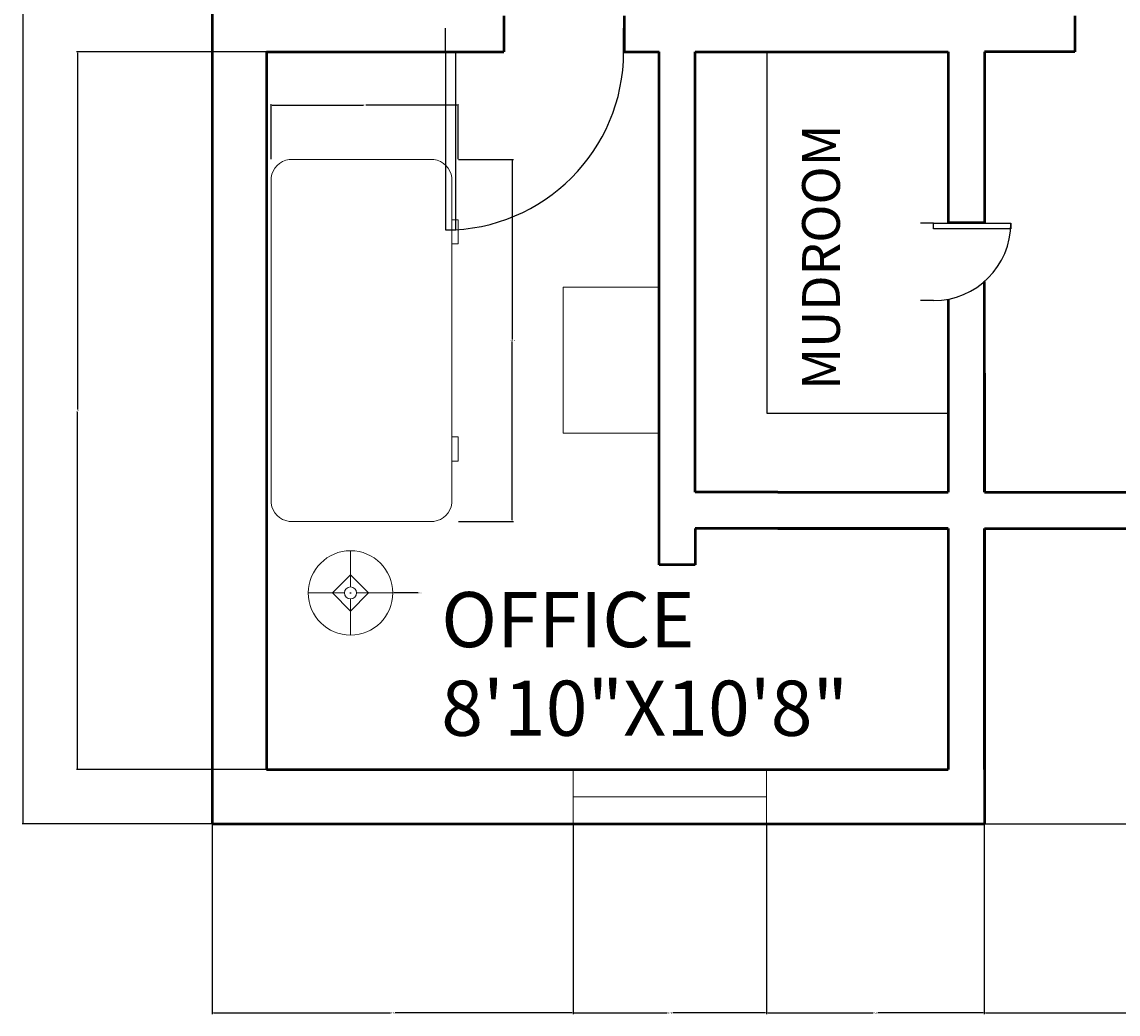
# Model space of a CAD drawing. Units: inches. Extents: x 2208 to 4689, y 1219 to 3512.
# Tile 1 of 5: x 2208 to 2389, y 1219 to 1383. Entities that reach past the tile are written whole.
import ezdxf

# ---------------------------------------------------------------- set-up
doc = ezdxf.new("R2010")
doc.units = ezdxf.units.IN
for name, color, linetype, lineweight in [('A-ANNO-DIMS', 2, 'Continuous', 18), ('A-AREA-IDEN', 7, 'Continuous', 18), ('A-DOOR', 3, 'Continuous', 25), ('A-FLOR-CASE', 9, 'Continuous', 25), ('A-FURN', 8, 'Continuous', 18), ('A-GLAZ', 4, 'Continuous', 18), ('A-WALL', 7, 'Continuous', 50)]:
    doc.layers.add(name, color=color, linetype=linetype, lineweight=lineweight)
doc.styles.get("Standard").update_dxf_attribs({"font": 'arial.ttf'})
doc.dimstyles.get("Standard").update_dxf_attribs({"dimtxt": 0.18, "dimasz": 0.18, "dimexe": 0.18, "dimexo": 0.0625, "dimgap": 0.09, "dimtad": 0, "dimtih": 1, "dimtoh": 1, "dimdec": 4, "dimzin": 0, "dimdsep": 46, "dimtxsty": 'Standard', "dimcen": 0.09, "dimadec": 0, "dimazin": 0, "dimtfac": 1, "dimtdec": 4, "dimtofl": 0, "dimtmove": 0, "dimatfit": 3, "dimfxl": 1, "dimtolj": 1, "dimtzin": 0, "dimarcsym": 0})

# ---------------------------------------------------------------- blocks, each defined once
blk = doc.blocks.new('*U15')
for p, q in [((0, 0), (0, -100)), ((600, 0), (600, -100))]:
    blk.add_line(p, q)
blk.add_lwpolyline([(0, 0), (0, 600), (43.75, 600), (43.75, 0)], close=True)
blk.add_arc((0, 0), 600, 0, 90)
blk = doc.blocks.new('Lamp - Table')
for p, q in [((0, 7), (0, 1)), ((0, 3), (-3, 0)), ((3, 0), (0, 3)), ((-1, 0), (-7, 0)), ((-3, 0), (0, -3)), ((0, -3), (3, 0)), ((1, 0), (7, 0)), ((0, -1), (0, -7))]:
    blk.add_line(p, q)
for radius in [7, 1]:
    blk.add_circle((0, 0), radius)
blk = doc.blocks.new('Desk - 30 x 60 in.')
for p, q in [((-26.999995, 0), (26.999995, 0)), ((-29.999995, -27), (-29.999995, -3)), ((29.999995, -3), (29.999995, -27)), ((26.999995, -30), (-26.999995, -30)), ((-20.000005, -30), (-20.000005, -31)), ((-16.000005, -31), (-16.000005, -30)), ((15.999995, -31), (15.999995, -30)), ((19.999995, -30), (19.999995, -31)), ((-20.000005, -31), (-16.000005, -31)), ((19.999995, -31), (15.999995, -31))]:
    blk.add_line(p, q)
for centre, start, end in [((-26.499995, -3.5), 98.1301, 171.8699), ((26.499995, -3.5), 8.130102, 81.8699), ((-26.499995, -26.5), 188.1301, 261.8699), ((26.499995, -26.5), 278.1301, 351.8699)]:
    blk.add_arc(centre, 3.535534, start, end)
blk = doc.blocks.new('*U4')
for p, q in [((0, 0), (0, 100)), ((750, 0), (750, 100))]:
    blk.add_line(p, q)
blk.add_lwpolyline([(0, 0), (0, -750), (43.75, -750), (43.75, 0)], close=True)
blk.add_arc((0, 0), 750, 270, 0)
blk = doc.blocks.new('*D26')
at = {"layer": 'A-ANNO-DIMS', "color": 0, "lineweight": -2, "transparency": 16777216}
for p, q in [((2279.91, 1360.51), (2289.03, 1360.51)), ((2288.85, 1360.33), (2288.85, 1330.69)), ((2288.85, 1300.69), (2288.85, 1330.32)), ((2279.91, 1300.51), (2289.03, 1300.51))]:
    blk.add_line(p, q, dxfattribs=at)
at = {"layer": 'A-ANNO-DIMS', "color": 0, "transparency": 16777216}
for points in [[(2288.82, 1360.33), (2288.88, 1360.33), (2288.85, 1360.51)], [(2288.82, 1300.69), (2288.88, 1300.69), (2288.85, 1300.51)]]:
    blk.add_solid(points, dxfattribs=at)
at = {"layer": 'Defpoints', "color": 0, "transparency": 16777216}
for p in [(2279.85, 1360.51), (2288.85, 1360.51), (2279.85, 1300.51)]:
    blk.add_point(p, dxfattribs=at)
at = {"layer": 'A-ANNO-DIMS', "color": 0, "transparency": 16777216, "insert": (2288.85, 1330.51), "char_height": 0.18, "attachment_point": 5}
blk.add_mtext('\\A1;DESK 60', dxfattribs=at)
blk = doc.blocks.new('*D27')
at = {"layer": 'A-ANNO-DIMS', "color": 0, "lineweight": -2, "transparency": 16777216}
for p, q in [((2248.85, 1360.57), (2248.85, 1369.69)), ((2249.03, 1369.51), (2264.15, 1369.51)), ((2279.67, 1369.51), (2264.55, 1369.51)), ((2279.85, 1360.57), (2279.85, 1369.69))]:
    blk.add_line(p, q, dxfattribs=at)
at = {"layer": 'A-ANNO-DIMS', "color": 0, "transparency": 16777216}
for points in [[(2249.03, 1369.54), (2249.03, 1369.48), (2248.85, 1369.51)], [(2279.67, 1369.54), (2279.67, 1369.48), (2279.85, 1369.51)]]:
    blk.add_solid(points, dxfattribs=at)
at = {"layer": 'Defpoints', "color": 0, "transparency": 16777216}
for p in [(2248.85, 1369.51), (2248.85, 1360.51), (2279.85, 1360.51)]:
    blk.add_point(p, dxfattribs=at)
at = {"layer": 'A-ANNO-DIMS', "color": 0, "transparency": 16777216, "insert": (2264.35, 1369.51), "char_height": 0.18, "attachment_point": 5}
blk.add_mtext('\\A1;31', dxfattribs=at)
blk = doc.blocks.new('*D35')
at = {"layer": 'A-ANNO-DIMS', "color": 0, "lineweight": -2, "transparency": 16777216}
for p, q in [((2239.04, 1850.36), (2207.57, 1850.36)), ((2207.75, 1850.18), (2207.75, 1550.54)), ((2207.75, 1250.54), (2207.75, 1550.17)), ((2239.04, 1250.36), (2207.57, 1250.36))]:
    blk.add_line(p, q, dxfattribs=at)
at = {"layer": 'A-ANNO-DIMS', "color": 0, "transparency": 16777216}
for points in [[(2207.72, 1850.18), (2207.78, 1850.18), (2207.75, 1850.36)], [(2207.72, 1250.54), (2207.78, 1250.54), (2207.75, 1250.36)]]:
    blk.add_solid(points, dxfattribs=at)
at = {"layer": 'Defpoints', "color": 0, "transparency": 16777216}
for p in [(2207.75, 1850.36), (2239.1, 1850.36), (2239.1, 1250.36)]:
    blk.add_point(p, dxfattribs=at)
at = {"layer": 'A-ANNO-DIMS', "color": 0, "transparency": 16777216, "insert": (2207.75, 1550.36), "char_height": 0.18, "attachment_point": 5}
blk.add_mtext('\\A1;600', dxfattribs=at)
blk = doc.blocks.new('*D40')
at = {"layer": 'A-ANNO-DIMS', "color": 0, "lineweight": -2, "transparency": 16777216}
for p, q in [((2248.04, 1378.36), (2216.57, 1378.36)), ((2216.75, 1378.18), (2216.75, 1319.04)), ((2216.75, 1259.54), (2216.75, 1318.67)), ((2248.04, 1259.36), (2216.57, 1259.36))]:
    blk.add_line(p, q, dxfattribs=at)
at = {"layer": 'A-ANNO-DIMS', "color": 0, "transparency": 16777216}
for points in [[(2216.72, 1378.18), (2216.78, 1378.18), (2216.75, 1378.36)], [(2216.72, 1259.54), (2216.78, 1259.54), (2216.75, 1259.36)]]:
    blk.add_solid(points, dxfattribs=at)
at = {"layer": 'Defpoints', "color": 0, "transparency": 16777216}
for p in [(2216.75, 1378.36), (2248.1, 1378.36), (2248.1, 1259.36)]:
    blk.add_point(p, dxfattribs=at)
at = {"layer": 'A-ANNO-DIMS', "color": 0, "transparency": 16777216, "insert": (2216.75, 1318.86), "char_height": 0.18, "attachment_point": 5}
blk.add_mtext('\\A1;119', dxfattribs=at)
blk = doc.blocks.new('*D47')
at = {"layer": 'A-ANNO-DIMS', "color": 0, "lineweight": -2, "transparency": 16777216}
for p, q in [((2239.1, 1250.29), (2239.1, 1218.83)), ((2298.94, 1250.29), (2298.94, 1218.83)), ((2239.28, 1219.01), (2268.63, 1219.01)), ((2298.76, 1219.01), (2269.41, 1219.01))]:
    blk.add_line(p, q, dxfattribs=at)
at = {"layer": 'A-ANNO-DIMS', "color": 0, "transparency": 16777216}
for points in [[(2239.28, 1219.04), (2239.28, 1218.98), (2239.1, 1219.01)], [(2298.76, 1219.04), (2298.76, 1218.98), (2298.94, 1219.01)]]:
    blk.add_solid(points, dxfattribs=at)
at = {"layer": 'Defpoints', "color": 0, "transparency": 16777216}
for p in [(2239.1, 1250.36), (2298.94, 1250.36), (2298.94, 1219.01)]:
    blk.add_point(p, dxfattribs=at)
at = {"layer": 'A-ANNO-DIMS', "color": 0, "transparency": 16777216, "insert": (2269.02, 1219.01), "char_height": 0.18, "attachment_point": 5}
blk.add_mtext('\\A1;59.84', dxfattribs=at)
blk = doc.blocks.new('*D48')
at = {"layer": 'A-ANNO-DIMS', "color": 0, "lineweight": -2, "transparency": 16777216}
for p, q in [((2298.94, 1250.29), (2298.94, 1218.83)), ((2331.01, 1250.29), (2331.01, 1218.83)), ((2299.12, 1219.01), (2314.51, 1219.01)), ((2330.83, 1219.01), (2315.44, 1219.01))]:
    blk.add_line(p, q, dxfattribs=at)
at = {"layer": 'A-ANNO-DIMS', "color": 0, "transparency": 16777216}
for points in [[(2299.12, 1219.04), (2299.12, 1218.98), (2298.94, 1219.01)], [(2330.83, 1219.04), (2330.83, 1218.98), (2331.01, 1219.01)]]:
    blk.add_solid(points, dxfattribs=at)
at = {"layer": 'Defpoints', "color": 0, "transparency": 16777216}
for p in [(2298.94, 1250.36), (2331.01, 1250.36), (2331.01, 1219.01)]:
    blk.add_point(p, dxfattribs=at)
at = {"layer": 'A-ANNO-DIMS', "color": 0, "transparency": 16777216, "insert": (2314.97, 1219.01), "char_height": 0.18, "attachment_point": 5}
blk.add_mtext('\\A1;32.064', dxfattribs=at)
blk = doc.blocks.new('*D49')
at = {"layer": 'A-ANNO-DIMS', "color": 0, "lineweight": -2, "transparency": 16777216}
for p, q in [((2331.01, 1250.29), (2331.01, 1218.83)), ((2367.11, 1250.29), (2367.11, 1218.83)), ((2331.19, 1219.01), (2348.68, 1219.01)), ((2366.93, 1219.01), (2349.44, 1219.01))]:
    blk.add_line(p, q, dxfattribs=at)
at = {"layer": 'A-ANNO-DIMS', "color": 0, "transparency": 16777216}
for points in [[(2331.19, 1219.04), (2331.19, 1218.98), (2331.01, 1219.01)], [(2366.93, 1219.04), (2366.93, 1218.98), (2367.11, 1219.01)]]:
    blk.add_solid(points, dxfattribs=at)
at = {"layer": 'Defpoints', "color": 0, "transparency": 16777216}
for p in [(2331.01, 1250.36), (2367.11, 1250.36), (2367.11, 1219.01)]:
    blk.add_point(p, dxfattribs=at)
at = {"layer": 'A-ANNO-DIMS', "color": 0, "transparency": 16777216, "insert": (2349.06, 1219.01), "char_height": 0.18, "attachment_point": 5}
blk.add_mtext('\\A1;36.11', dxfattribs=at)
blk = doc.blocks.new('*D50')
at = {"layer": 'A-ANNO-DIMS', "color": 0, "lineweight": -2, "transparency": 16777216}
for p, q in [((2367.11, 1299.29), (2367.11, 1218.83)), ((2427.95, 1299.29), (2427.95, 1218.83)), ((2367.29, 1219.01), (2397.14, 1219.01)), ((2427.77, 1219.01), (2397.93, 1219.01))]:
    blk.add_line(p, q, dxfattribs=at)
at = {"layer": 'A-ANNO-DIMS', "color": 0, "transparency": 16777216}
for points in [[(2367.29, 1219.04), (2367.29, 1218.98), (2367.11, 1219.01)], [(2427.77, 1219.04), (2427.77, 1218.98), (2427.95, 1219.01)]]:
    blk.add_solid(points, dxfattribs=at)
at = {"layer": 'Defpoints', "color": 0, "transparency": 16777216}
for p in [(2367.11, 1299.36), (2427.95, 1299.36), (2427.95, 1219.01)]:
    blk.add_point(p, dxfattribs=at)
at = {"layer": 'A-ANNO-DIMS', "color": 0, "transparency": 16777216, "insert": (2397.53, 1219.01), "char_height": 0.18, "attachment_point": 5}
blk.add_mtext('\\A1;60.84', dxfattribs=at)
blk = doc.blocks.new('*D54')
at = {"layer": 'A-ANNO-DIMS', "color": 0, "lineweight": -2, "transparency": 16777216}
for p, q in [((2367.18, 1299.36), (2684.63, 1299.36)), ((2684.45, 1299.18), (2684.45, 1275.04)), ((2684.45, 1250.54), (2684.45, 1274.67)), ((2367.18, 1250.36), (2684.63, 1250.36))]:
    blk.add_line(p, q, dxfattribs=at)
at = {"layer": 'A-ANNO-DIMS', "color": 0, "transparency": 16777216}
for points in [[(2684.42, 1299.18), (2684.48, 1299.18), (2684.45, 1299.36)], [(2684.42, 1250.54), (2684.48, 1250.54), (2684.45, 1250.36)]]:
    blk.add_solid(points, dxfattribs=at)
at = {"layer": 'Defpoints', "color": 0, "transparency": 16777216}
for p in [(2367.11, 1299.36), (2684.45, 1299.36), (2367.11, 1250.36)]:
    blk.add_point(p, dxfattribs=at)
at = {"layer": 'A-ANNO-DIMS', "color": 0, "transparency": 16777216, "insert": (2684.45, 1274.86), "char_height": 0.18, "attachment_point": 5}
blk.add_mtext('\\A1;49', dxfattribs=at)
blk = doc.blocks.new('*D75')
at = {"layer": 'A-ANNO-DIMS', "color": 0, "lineweight": -2, "transparency": 16777216}
for p, q in [((2261.94, 1288.65), (2262.12, 1288.65)), ((2262.03, 1288.56), (2262.03, 1288.74)), ((2273.23, 1288.65), (2269.21, 1288.65))]:
    blk.add_line(p, q, dxfattribs=at)
at = {"layer": 'A-ANNO-DIMS', "color": 0, "transparency": 16777216}
blk.add_solid([(2269.21, 1288.68), (2269.21, 1288.62), (2269.03, 1288.65)], dxfattribs=at)
at = {"layer": 'Defpoints', "color": 0, "transparency": 16777216}
for p in [(2255.03, 1288.65), (2269.03, 1288.65)]:
    blk.add_point(p, dxfattribs=at)
at = {"layer": 'A-ANNO-DIMS', "color": 0, "transparency": 16777216, "insert": (2273.54, 1288.65), "char_height": 0.18, "attachment_point": 5}
blk.add_mtext('\\A1;∅14', dxfattribs=at)

msp = doc.modelspace()

# ---------------------------------------------------------------- linework, layer by layer
at = {"layer": 'A-FLOR-CASE'}
for p, q in [((2331.0555, 1378.3551), (2331.0555, 1318.4467)), ((2331.0555, 1318.4467), (2361.1139, 1318.4467))]:
    msp.add_line(p, q, dxfattribs=at)
at = {"layer": 'A-FURN'}
msp.add_lwpolyline([(2297.2741, 1339.35), (2313.177, 1339.35), (2313.177, 1315.1467), (2297.2741, 1315.1467)], close=True, dxfattribs=at)
at = {"layer": 'A-GLAZ'}
for p, q in [((2298.9423, 1254.8551), (2298.9423, 1259.3551)), ((2298.9423, 1259.3551), (2298.9423, 1250.3551)), ((2331.0059, 1259.3551), (2331.0059, 1250.3551)), ((2331.0059, 1254.8551), (2298.9423, 1254.8551)), ((2331.0059, 1250.3551), (2331.0059, 1254.8551))]:
    msp.add_line(p, q, dxfattribs=at)
at = {"layer": 'A-WALL'}
for p, q in [((2239.0983, 1850.3551), (2239.0983, 1250.3551)), ((2287.452, 1384.3551), (2287.452, 1378.3551)), ((2307.3743, 1384.3551), (2307.3743, 1378.3551)), ((2382.135, 1384.3551), (2382.135, 1378.3551)), ((2248.0983, 1378.3551), (2283.3743, 1378.3551)), ((2248.0983, 1378.3551), (2283.3743, 1378.3551)), ((2248.0983, 1378.3551), (2283.3743, 1378.3551)), ((2248.0983, 1378.3551), (2248.0983, 1259.3551)), ((2283.3743, 1378.3551), (2287.452, 1378.3551)), ((2307.3743, 1378.3551), (2313.177, 1378.3551)), ((2307.3743, 1378.3551), (2313.177, 1378.3551)), ((2307.3743, 1378.3551), (2313.177, 1378.3551)), ((2313.177, 1299.3551), (2313.177, 1378.3551)), ((2319.177, 1305.3551), (2319.177, 1378.3551)), ((2319.177, 1378.3551), (2361.1139, 1378.3551)), ((2319.177, 1378.3551), (2361.1139, 1378.3551)), ((2319.177, 1378.3551), (2347.7152, 1378.3551)), ((2361.1139, 1378.3551), (2361.1139, 1350.0584)), ((2367.1139, 1378.3551), (2367.1139, 1350.0584)), ((2382.135, 1378.3551), (2367.1139, 1378.3551)), ((2361.1139, 1350.0584), (2367.1139, 1350.0584)), ((2367.1139, 1305.3551), (2367.1139, 1340.2706)), ((2361.1139, 1337.3443), (2361.1139, 1305.3551)), ((2367.1139, 1325.0806), (2367.1139, 1305.3551)), ((2332.8555, 1305.3551), (2319.177, 1305.3551)), ((2332.8555, 1305.3551), (2361.1139, 1305.3551)), ((2367.1139, 1305.3551), (2520.2866, 1305.3551)), ((2313.177, 1293.3068), (2313.177, 1299.3551)), ((2332.8555, 1299.3551), (2319.177, 1299.3551)), ((2319.177, 1299.3551), (2319.177, 1293.3068)), ((2361.1139, 1299.3551), (2332.8555, 1299.3551)), ((2332.8555, 1299.3551), (2361.1139, 1299.3551)), ((2361.1139, 1299.3551), (2361.1139, 1259.3551)), ((2367.1139, 1259.3551), (2367.1139, 1299.3551)), ((2367.1139, 1299.3551), (2526.2866, 1299.3551)), ((2367.1139, 1299.3551), (2367.1139, 1259.3551)), ((2319.177, 1293.3068), (2313.177, 1293.3068)), ((2248.0983, 1259.3551), (2361.1139, 1259.3551)), ((2367.1139, 1259.3551), (2367.1139, 1250.3551)), ((2239.0983, 1250.3551), (2367.1139, 1250.3551))]:
    msp.add_line(p, q, dxfattribs=at)

# ---------------------------------------------------------------- block references
at = {"layer": 'A-DOOR', "xscale": 0.0393700787401575, "yscale": 0.0393700787401575, "zscale": 0.0393700787401575}
msp.add_blockref('*U4', (2277.7765, 1378.3551), dxfattribs=at)
at = {"layer": 'A-DOOR', "xscale": 0.0213818566096311, "yscale": 0.0213818566096311, "zscale": 0.0213818566096311, "rotation": 270}
msp.add_blockref('*U15', (2358.6838, 1349.9411), dxfattribs=at)
at = {"layer": 'A-FURN', "rotation": 90}
msp.add_blockref('Desk - 30 x 60 in.', (2248.8474, 1330.508), dxfattribs=at)
at = {"layer": 'A-FURN'}
msp.add_blockref('Lamp - Table', (2262.0285, 1288.6486), dxfattribs=at)

# ---------------------------------------------------------------- texts
at = {"layer": 'A-AREA-IDEN'}
msp.add_text('MUDROOM', height=6.25599, rotation=90, dxfattribs=at).set_placement((2343.1568, 1322.3402))
for s, p in [('OFFICE', (2277.0677, 1279.654)), ('8\'10"X10\'8"', (2277.0677, 1264.9619))]:
    msp.add_text(s, height=9.14594, dxfattribs=at).set_placement(p)

# ---------------------------------------------------------------- dimensions: what is measured, and where the dimension line sits
at = {"layer": 'A-ANNO-DIMS'}
for base, p1, p2, angle, picture, middle in [((2207.7483, 1850.3551), (2239.0983, 1250.3551), (2239.0983, 1850.3551), 90, '*D35', (2207.7483, 1550.3551)), ((2216.7483, 1378.3551), (2248.0983, 1259.3551), (2248.0983, 1378.3551), 90, '*D40', (2216.7483, 1318.8551)), ((2248.8474, 1369.508), (2279.8474, 1360.508), (2248.8474, 1360.508), 180, '*D27', (2264.3474, 1369.508)), ((2684.4483, 1299.3551), (2367.1139, 1250.3551), (2367.1139, 1299.3551), 90, '*D54', (2684.4483, 1274.8551))]:
    dim = msp.add_linear_dim(base=base, p1=p1, p2=p2, angle=angle, dimstyle='Standard', override={"dimdec": 0, "dimlfac": 1, "dimrnd": 0, "dimzin": 0, "dimdsep": 46, "dimlunit": 2}, dxfattribs=at)
    dim.commit()
    dim.dimension.update_dxf_attribs({"geometry": picture, "text_midpoint": middle})
dim = msp.add_linear_dim(base=(2288.8474, 1360.508), p1=(2279.8474, 1300.508), p2=(2279.8474, 1360.508), angle=90, text='DESK <>', dimstyle='Standard', override={"dimdec": 0, "dimlfac": 1, "dimrnd": 0, "dimzin": 0, "dimdsep": 46, "dimlunit": 2}, dxfattribs=at)
dim.commit()
dim.dimension.update_dxf_attribs({"geometry": '*D26', "text_midpoint": (2288.8474, 1330.508)})
for base, p1, p2, override, picture, middle in [((2427.9528, 1219.0051), (2367.1139, 1299.3551), (2427.9528, 1299.3551), {"dimdec": 2, "dimlfac": 1, "dimrnd": 0, "dimzin": 0, "dimdsep": 46, "dimlunit": 2}, '*D50', (2397.5333, 1219.0051)), ((2298.9423, 1219.0051), (2239.0983, 1250.3551), (2298.9423, 1250.3551), {"dimdec": 2, "dimlfac": 1, "dimrnd": 0, "dimzin": 0, "dimdsep": 46, "dimlunit": 2}, '*D47', (2269.0203, 1219.0051)), ((2331.0059, 1219.0051), (2298.9423, 1250.3551), (2331.0059, 1250.3551), {"dimdec": 3, "dimlfac": 1, "dimrnd": 0, "dimzin": 0, "dimdsep": 46, "dimlunit": 2}, '*D48', (2314.9741, 1219.0051)), ((2367.1139, 1219.0051), (2331.0059, 1250.3551), (2367.1139, 1250.3551), {"dimdec": 2, "dimlfac": 1, "dimrnd": 0, "dimzin": 0, "dimdsep": 46, "dimlunit": 2}, '*D49', (2349.0599, 1219.0051))]:
    dim = msp.add_linear_dim(base=base, p1=p1, p2=p2, dimstyle='Standard', override=override, dxfattribs=at)
    dim.commit()
    dim.dimension.update_dxf_attribs({"geometry": picture, "text_midpoint": middle})
dim = msp.add_diameter_dim_2p(p1=(2255.0285, 1288.6481), p2=(2269.0285, 1288.649), dimstyle='Standard', override={"dimdec": 0, "dimlfac": 1, "dimrnd": 0, "dimzin": 0, "dimdsep": 46, "dimlunit": 2}, dxfattribs=at)
dim.commit()
dim.dimension.update_dxf_attribs({"geometry": '*D75', "text_midpoint": (2273.2285, 1288.6493), "dimtype": 163})

doc.saveas('drawing.dxf')
